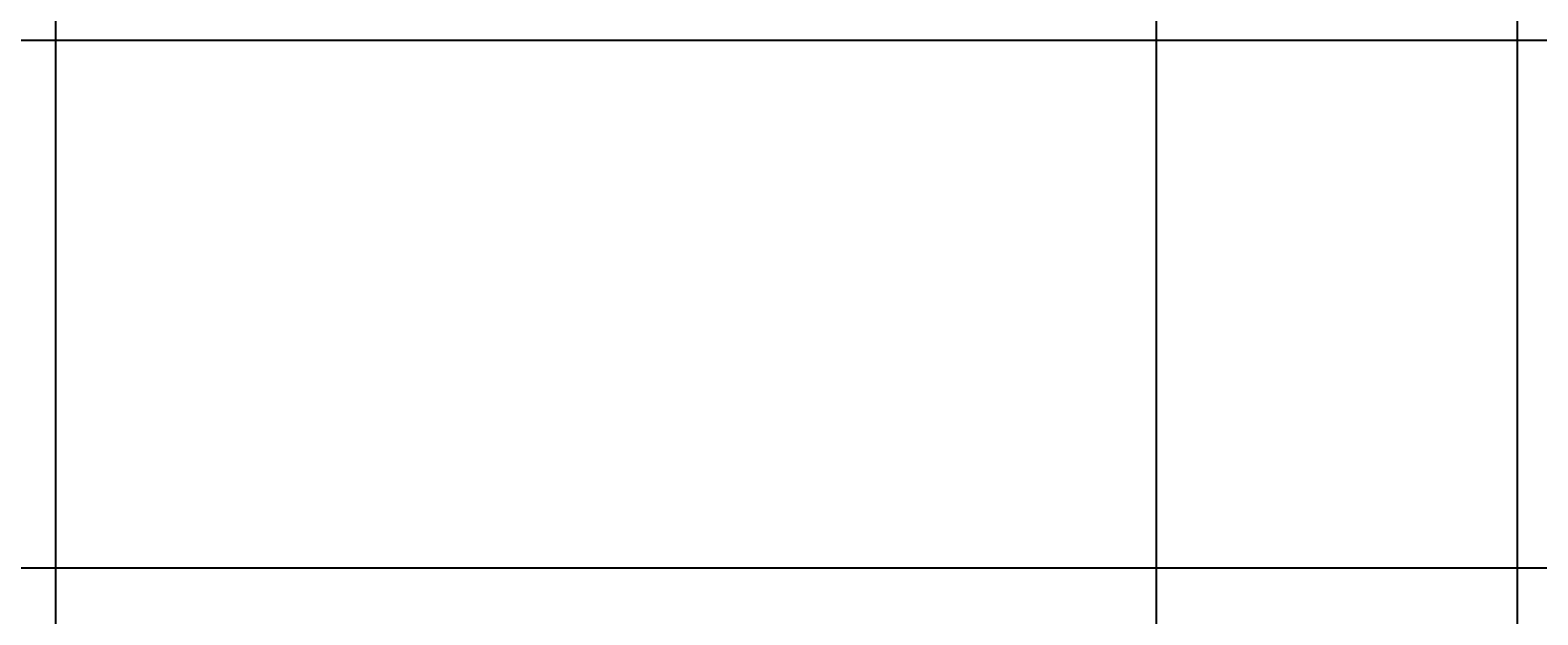
# Model space of a CAD drawing. Units: inches. Extents: x 35362 to 73946, y 43607 to 67532.
# Tile 56 of 134: x 50119 to 51337, y 46091 to 46564. Entities that reach past the tile are written whole.
import ezdxf

# ---------------------------------------------------------------- set-up
doc = ezdxf.new("R2010")
doc.units = ezdxf.units.IN
doc.header["$MEASUREMENT"] = 0
doc.layers.add('A-ANNO-DIMS', color=2, linetype='Continuous', lineweight=18)
doc.styles.get("Standard").update_dxf_attribs({"font": 'arial.ttf'})
doc.dimstyles.get("Standard").update_dxf_attribs({"dimtxt": 0.18, "dimasz": 0.18, "dimexe": 0.18, "dimexo": 0.0625, "dimgap": 0.09, "dimtad": 0, "dimtih": 1, "dimtoh": 1, "dimdec": 4, "dimzin": 0, "dimdsep": 46, "dimtxsty": 'Standard', "dimcen": 0.09, "dimadec": 0, "dimazin": 0, "dimtfac": 1, "dimtdec": 4, "dimtofl": 0, "dimtmove": 0, "dimatfit": 3, "dimfxl": 1, "dimtolj": 1, "dimtzin": 0, "dimarcsym": 0})

# ---------------------------------------------------------------- blocks, each defined once
blk = doc.blocks.new('*D5')
at = {"layer": 'A-ANNO-DIMS', "color": 0, "lineweight": -2, "transparency": 16777216}
for p, q in [((37121.9, 46919.3), (37121.9, 43606.7)), ((69871.5, 45449.8), (69871.5, 43606.7)), ((37122.1, 43606.9), (53496.3, 43606.9)), ((69871.3, 43606.9), (53497.2, 43606.9))]:
    blk.add_line(p, q, dxfattribs=at)
at = {"layer": 'A-ANNO-DIMS', "color": 0, "transparency": 16777216}
for points in [[(37122.1, 43606.9), (37122.1, 43606.8), (37121.9, 43606.9)], [(69871.3, 43606.9), (69871.3, 43606.8), (69871.5, 43606.9)]]:
    blk.add_solid(points, dxfattribs=at)
at = {"layer": 'Defpoints', "color": 0, "transparency": 16777216}
for p in [(37121.9, 46919.4), (69871.5, 45449.9), (69871.5, 43606.9)]:
    blk.add_point(p, dxfattribs=at)
at = {"layer": 'A-ANNO-DIMS', "color": 0, "transparency": 16777216, "insert": (53496.7, 43606.9), "char_height": 0.18, "attachment_point": 5}
blk.add_mtext('\\A1;32750', dxfattribs=at)
blk = doc.blocks.new('*D11')
at = {"layer": 'A-ANNO-DIMS', "color": 0, "lineweight": -2, "transparency": 16777216}
for p, q in [((47978.7, 56028.8), (47978.7, 43606.7)), ((53109.8, 56028.8), (53109.8, 43606.7)), ((47978.8, 43606.9), (50543.9, 43606.9)), ((53109.6, 43606.9), (50544.6, 43606.9))]:
    blk.add_line(p, q, dxfattribs=at)
at = {"layer": 'A-ANNO-DIMS', "color": 0, "transparency": 16777216}
for points in [[(47978.8, 43606.9), (47978.8, 43606.8), (47978.7, 43606.9)], [(53109.6, 43606.9), (53109.6, 43606.8), (53109.8, 43606.9)]]:
    blk.add_solid(points, dxfattribs=at)
at = {"layer": 'Defpoints', "color": 0, "transparency": 16777216}
for p in [(47978.7, 56028.8), (53109.8, 56028.8), (53109.8, 43606.9)]:
    blk.add_point(p, dxfattribs=at)
at = {"layer": 'A-ANNO-DIMS', "color": 0, "transparency": 16777216, "insert": (50544.2, 43606.9), "char_height": 0.18, "attachment_point": 5}
blk.add_mtext('\\A1;5131', dxfattribs=at)
blk = doc.blocks.new('*D13')
at = {"layer": 'A-ANNO-DIMS', "color": 0, "lineweight": -2, "transparency": 16777216}
for p, q in [((48373.5, 51694), (48373.5, 43606.7)), ((51029, 51694), (51029, 43606.7)), ((48373.7, 43606.9), (49700.8, 43606.9)), ((51028.9, 43606.9), (49701.7, 43606.9))]:
    blk.add_line(p, q, dxfattribs=at)
at = {"layer": 'A-ANNO-DIMS', "color": 0, "transparency": 16777216}
for points in [[(48373.7, 43606.9), (48373.7, 43606.8), (48373.5, 43606.9)], [(51028.9, 43606.9), (51028.9, 43606.8), (51029, 43606.9)]]:
    blk.add_solid(points, dxfattribs=at)
at = {"layer": 'Defpoints', "color": 0, "transparency": 16777216}
for p in [(48373.5, 51694.1), (51029, 51694.1), (51029, 43606.9)]:
    blk.add_point(p, dxfattribs=at)
at = {"layer": 'A-ANNO-DIMS', "color": 0, "transparency": 16777216, "insert": (49701.3, 43606.9), "char_height": 0.18, "attachment_point": 5}
blk.add_mtext('\\A1;2655.6', dxfattribs=at)
blk = doc.blocks.new('*D17')
at = {"layer": 'A-ANNO-DIMS', "color": 0, "lineweight": -2, "transparency": 16777216}
for p, q in [((49923.3, 61293.2), (49923.3, 43606.7)), ((51913.9, 61293.2), (51913.9, 43606.7)), ((49923.5, 43606.9), (50918.2, 43606.9)), ((51913.8, 43606.9), (50919.1, 43606.9))]:
    blk.add_line(p, q, dxfattribs=at)
at = {"layer": 'A-ANNO-DIMS', "color": 0, "transparency": 16777216}
for points in [[(49923.5, 43606.9), (49923.5, 43606.8), (49923.3, 43606.9)], [(51913.8, 43606.9), (51913.8, 43606.8), (51913.9, 43606.9)]]:
    blk.add_solid(points, dxfattribs=at)
at = {"layer": 'Defpoints', "color": 0, "transparency": 16777216}
for p in [(49923.3, 61293.3), (51913.9, 61293.3), (51913.9, 43606.9)]:
    blk.add_point(p, dxfattribs=at)
at = {"layer": 'A-ANNO-DIMS', "color": 0, "transparency": 16777216, "insert": (50918.6, 43606.9), "char_height": 0.18, "attachment_point": 5}
blk.add_mtext('\\A1;1990.6', dxfattribs=at)
blk = doc.blocks.new('*D67')
at = {"layer": 'A-ANNO-DIMS', "color": 0, "lineweight": -2, "transparency": 16777216}
for p, q in [((56873.5, 53351.5), (35361.8, 53351.5)), ((35361.9, 53351.3), (35361.9, 49400.9)), ((35361.9, 45450.1), (35361.9, 49400.5)), ((53793.6, 45449.9), (35361.8, 45449.9))]:
    blk.add_line(p, q, dxfattribs=at)
at = {"layer": 'A-ANNO-DIMS', "color": 0, "transparency": 16777216}
for points in [[(35361.9, 53351.3), (35362, 53351.3), (35361.9, 53351.5)], [(35361.9, 45450.1), (35362, 45450.1), (35361.9, 45449.9)]]:
    blk.add_solid(points, dxfattribs=at)
at = {"layer": 'Defpoints', "color": 0, "transparency": 16777216}
for p in [(35361.9, 53351.5), (56873.6, 53351.5), (53793.6, 45449.9)]:
    blk.add_point(p, dxfattribs=at)
at = {"layer": 'A-ANNO-DIMS', "color": 0, "transparency": 16777216, "insert": (35361.9, 49400.7), "char_height": 0.18, "attachment_point": 5}
blk.add_mtext('\\A1;7901.6', dxfattribs=at)
blk = doc.blocks.new('*D76')
at = {"layer": 'A-ANNO-DIMS', "color": 0, "lineweight": -2, "transparency": 16777216}
for p, q in [((54052.8, 46555.3), (35361.8, 46555.3)), ((35361.9, 46555.1), (35361.9, 46342.3)), ((35361.9, 46129.1), (35361.9, 46341.9)), ((53793.6, 46128.9), (35361.8, 46128.9))]:
    blk.add_line(p, q, dxfattribs=at)
at = {"layer": 'A-ANNO-DIMS', "color": 0, "transparency": 16777216}
for points in [[(35361.9, 46555.1), (35362, 46555.1), (35361.9, 46555.3)], [(35361.9, 46129.1), (35362, 46129.1), (35361.9, 46128.9)]]:
    blk.add_solid(points, dxfattribs=at)
at = {"layer": 'Defpoints', "color": 0, "transparency": 16777216}
for p in [(35361.9, 46555.3), (54052.9, 46555.3), (53793.6, 46128.9)]:
    blk.add_point(p, dxfattribs=at)
at = {"layer": 'A-ANNO-DIMS', "color": 0, "transparency": 16777216, "insert": (35361.9, 46342.1), "char_height": 0.18, "attachment_point": 5}
blk.add_mtext('\\A1;426.4', dxfattribs=at)
blk = doc.blocks.new('*D90')
at = {"layer": 'A-ANNO-DIMS', "color": 0, "lineweight": -2, "transparency": 16777216}
for p, q in [((53707.7, 47291.3), (35361.8, 47291.3)), ((35361.9, 47291.1), (35361.9, 46710.3)), ((35361.9, 46129.1), (35361.9, 46709.9)), ((53793.6, 46128.9), (35361.8, 46128.9))]:
    blk.add_line(p, q, dxfattribs=at)
at = {"layer": 'A-ANNO-DIMS', "color": 0, "transparency": 16777216}
for points in [[(35361.9, 47291.1), (35362, 47291.1), (35361.9, 47291.3)], [(35361.9, 46129.1), (35362, 46129.1), (35361.9, 46128.9)]]:
    blk.add_solid(points, dxfattribs=at)
at = {"layer": 'Defpoints', "color": 0, "transparency": 16777216}
for p in [(53707.8, 47291.3), (35361.9, 46128.9), (53793.6, 46128.9)]:
    blk.add_point(p, dxfattribs=at)
at = {"layer": 'A-ANNO-DIMS', "color": 0, "transparency": 16777216, "insert": (35361.9, 46710.1), "char_height": 0.18, "attachment_point": 5}
blk.add_mtext('\\A1;1162.4', dxfattribs=at)
blk = doc.blocks.new('*D107')
at = {"layer": 'A-ANNO-DIMS', "color": 0, "lineweight": -2, "transparency": 16777216}
for p, q in [((50139.6, 59850), (50139.6, 43606.7)), ((51320.8, 59850), (51320.8, 43606.7)), ((50139.7, 43606.9), (50729.7, 43606.9)), ((51320.6, 43606.9), (50730.6, 43606.9))]:
    blk.add_line(p, q, dxfattribs=at)
at = {"layer": 'A-ANNO-DIMS', "color": 0, "transparency": 16777216}
for points in [[(50139.7, 43606.9), (50139.7, 43606.8), (50139.6, 43606.9)], [(51320.6, 43606.9), (51320.6, 43606.8), (51320.8, 43606.9)]]:
    blk.add_solid(points, dxfattribs=at)
at = {"layer": 'Defpoints', "color": 0, "transparency": 16777216}
for p in [(50139.6, 59850.1), (51320.8, 59850.1), (51320.8, 43606.9)]:
    blk.add_point(p, dxfattribs=at)
at = {"layer": 'A-ANNO-DIMS', "color": 0, "transparency": 16777216, "insert": (50730.2, 43606.9), "char_height": 0.18, "attachment_point": 5}
blk.add_mtext('\\A1;1181.3', dxfattribs=at)

msp = doc.modelspace()

# ---------------------------------------------------------------- dimensions: what is measured, and where the dimension line sits
at = {"layer": 'A-ANNO-DIMS'}
for base, p1, p2, override, picture, middle in [((51913.931, 43606.859), (49923.307, 61293.286), (51913.931, 61293.286), {"dimdec": 1, "dimlfac": 1, "dimrnd": 0, "dimzin": 0, "dimdsep": 46, "dimlunit": 2}, '*D17', (50918.619, 43606.859)), ((51320.8133, 43606.859), (50139.5627, 59850.0769), (51320.8133, 59850.0769), {"dimdec": 1, "dimlfac": 1, "dimrnd": 0, "dimzin": 0, "dimdsep": 46, "dimlunit": 2}, '*D107', (50730.188, 43606.859)), ((53109.76, 43606.859), (47978.665, 56028.836), (53109.76, 56028.836), {"dimdec": 0, "dimlfac": 1, "dimrnd": 0, "dimzin": 0, "dimdsep": 46, "dimlunit": 2}, '*D11', (50544.212, 43606.859)), ((51029.043, 43606.859), (48373.492, 51694.087), (51029.043, 51694.087), {"dimdec": 1, "dimlfac": 1, "dimrnd": 0, "dimzin": 0, "dimdsep": 46, "dimlunit": 2}, '*D13', (49701.267, 43606.859)), ((69871.496, 43606.859), (37121.949, 46919.381), (69871.496, 45449.894), {"dimdec": 0, "dimlfac": 1, "dimrnd": 0, "dimzin": 0, "dimdsep": 46, "dimlunit": 2}, '*D5', (53496.723, 43606.859))]:
    dim = msp.add_linear_dim(base=base, p1=p1, p2=p2, dimstyle='Standard', override=override, dxfattribs=at)
    dim.commit()
    dim.dimension.update_dxf_attribs({"geometry": picture, "text_midpoint": middle})
for base, p1, p2, picture, middle in [((35361.949, 53351.529), (53793.638, 45449.894), (56873.602, 53351.529), '*D67', (35361.949, 49400.712)), ((35361.949, 46128.878), (53707.781, 47291.285), (53793.638, 46128.878), '*D90', (35361.949, 46710.081)), ((35361.949, 46555.293), (53793.638, 46128.878), (54052.899, 46555.293), '*D76', (35361.949, 46342.086))]:
    dim = msp.add_linear_dim(base=base, p1=p1, p2=p2, angle=90, dimstyle='Standard', override={"dimdec": 1, "dimlfac": 1, "dimrnd": 0, "dimzin": 0, "dimdsep": 46, "dimlunit": 2}, dxfattribs=at)
    dim.commit()
    dim.dimension.update_dxf_attribs({"geometry": picture, "text_midpoint": middle})

doc.saveas('drawing.dxf')
